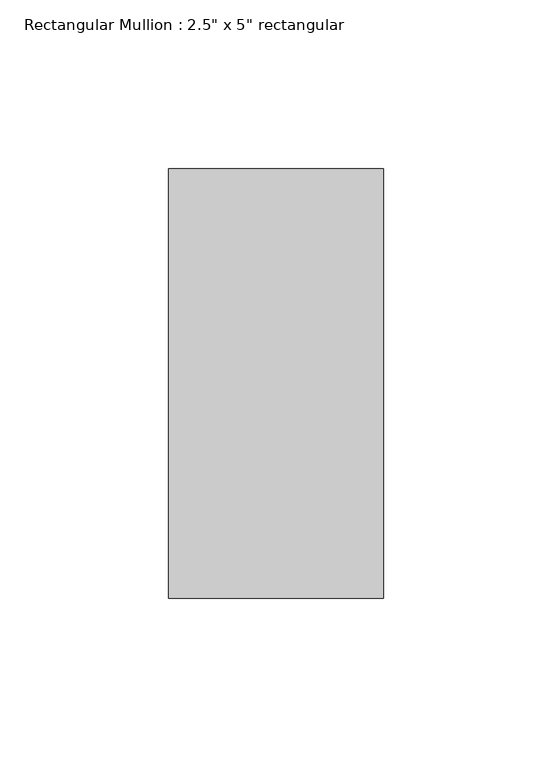
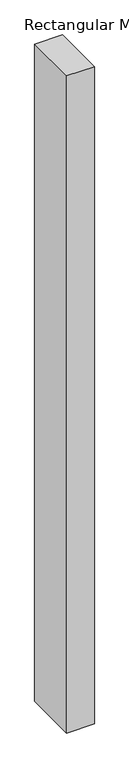
"""IFC4 building model written with IfcOpenShell, lengths in millimetres: member geometry."""

from ifc_helpers import new_model, si_unit, frame, origin, place, context, project, spatial, polyline, outline, extrude, source, transform, mapped, element, save


def member_3005f220(model_context):
    return source(origin(), model_context, "Body", "SweptSolid", [
        extrude(outline(polyline([(31.75, 63.5), (31.75, -63.5), (-31.75, -63.5), (-31.75, 63.5), (31.75, 63.5)])), frame((0.0, 0.0, -1593.034917), z_axis=(0.0, 0.0, 1.0), x_axis=(1.0, 0.0, 0.0)), (0.0, 0.0, 1.0), 1593.034917),
    ])


if __name__ == "__main__":
    model = new_model("IFC4")
    model_context = context("Model", 3, world=origin())
    ifc_project = project(units=[si_unit("LENGTHUNIT", "METRE", prefix="MILLI")], contexts=[model_context])
    site = spatial("IfcSite", under=ifc_project)
    building = spatial("IfcBuilding", under=site)
    placement = place(None, origin())
    member_shape = member_3005f220(model_context)
    element("IfcMember", 1, ObjectType="Rectangular Mullion : 2.5\" x 5\" rectangular", at=placement, inside=building, context=model_context, shape_type="MappedRepresentation", body=[
        mapped(member_shape, transform((0.0, 0.0, 0.0), x_axis=(1.0, 0.0, 0.0), y_axis=(0.0, 1.0, 0.0), z_axis=(0.0, 0.0, 1.0))),
    ])
    save(model, "model.ifc")

# Revit data of these elements
# Type "Rectangular Mullion : 2.5\" x 5\" rectangular"
#   built-in parameter 1007304 = 0.416667 (stored number, unit not read)
#   built-in parameter 1007301 = 0.104167 (stored number, unit not read)
#   built-in parameter 1007300 = 0.104167 (stored number, unit not read)
# Element 1 (IfcMember, "Rectangular Mullion : 2.5\" x 5\" rectangular")
#   Materials on its faces: "Aluminum"
# Materials
#   "Aluminum": class "Metal", colour RGB 247 247 247, transparency 0, Description = "Aluminum 6061", Cost = 0
